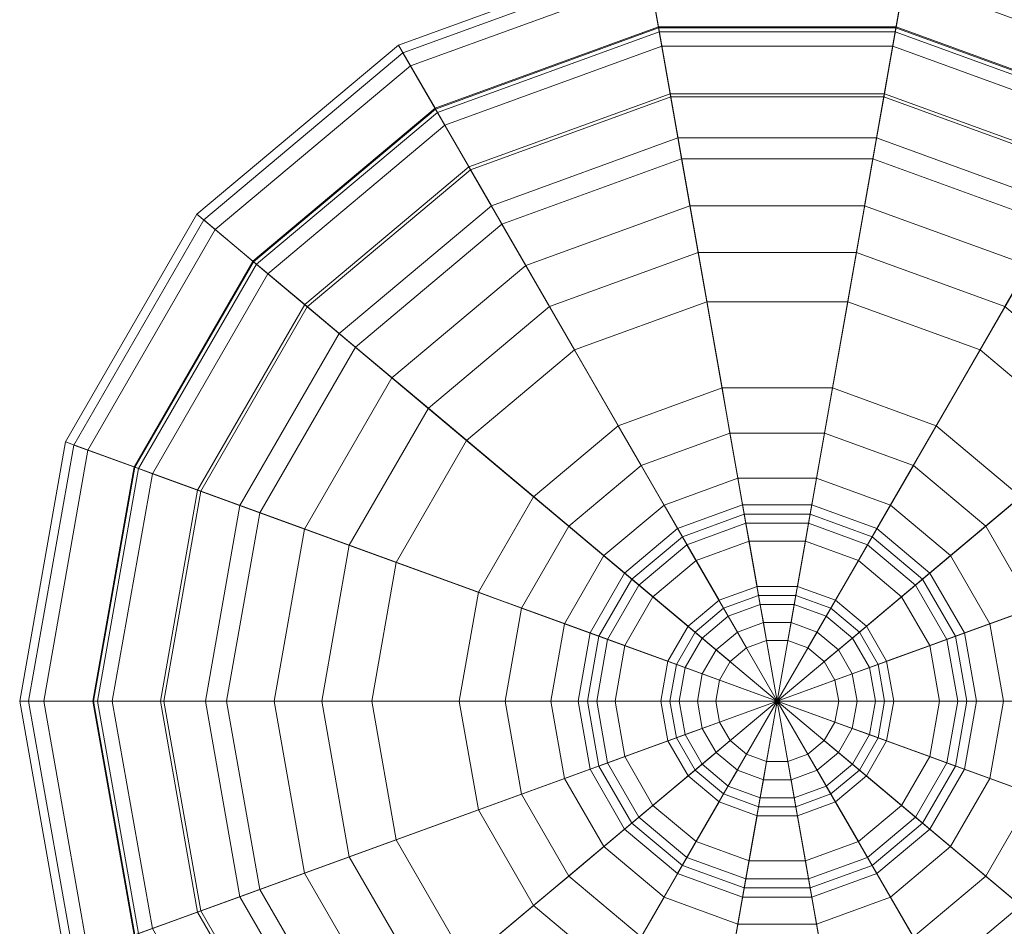
# Model space of a CAD drawing. Units: inches. Extents: x 375 to 1122, y 27 to 1069.
# Tile 42 of 155: x 717.909 to 719.669, y 298.684 to 300.305. Entities that reach past the tile are written whole.
import ezdxf

# ---------------------------------------------------------------- set-up
doc = ezdxf.new("R2010")
doc.units = ezdxf.units.IN
doc.layers.add('Furniture', color=30, linetype='Continuous', lineweight=18)

# ---------------------------------------------------------------- blocks, each defined once
blk = doc.blocks.new('A$C403C54AD')
for points in [[(1.180252, 0.891746, -0.031825), (1.180252, 0.857884, -0.028747), (1.180252, 0.857884, -0.028747), (1.16867, 0.889704, -0.031825)], [(1.191834, 0.889704, -0.031825), (1.180252, 0.857884, -0.028747), (1.180252, 0.857884, -0.028747), (1.180252, 0.891746, -0.031825)], [(1.16867, 0.889704, -0.031825), (1.180252, 0.857884, -0.028747), (1.180252, 0.857884, -0.028747), (1.158486, 0.883824, -0.031825)], [(1.202018, 0.883824, -0.031825), (1.180252, 0.857884, -0.028747), (1.180252, 0.857884, -0.028747), (1.191834, 0.889704, -0.031825)], [(1.158486, 0.883824, -0.031825), (1.180252, 0.857884, -0.028747), (1.180252, 0.857884, -0.028747), (1.150927, 0.874815, -0.031825)], [(1.209578, 0.874815, -0.031825), (1.180252, 0.857884, -0.028747), (1.180252, 0.857884, -0.028747), (1.202018, 0.883824, -0.031825)], [(1.171115, 0.868773, -0.02532), (1.160585, 0.881322, -0.028594), (1.153755, 0.873182, -0.028594), (1.167942, 0.864991, -0.02532)], [(1.192562, 0.864991, -0.02532), (1.206749, 0.873182, -0.028594), (1.199919, 0.881322, -0.028594), (1.189389, 0.868773, -0.02532)], [(1.180252, 0.878242, 0.061451), (1.180252, 0.868003, 0.054084), (1.176791, 0.867392, 0.054084), (1.173289, 0.877014, 0.061451)], [(1.187215, 0.877014, 0.061451), (1.183713, 0.867392, 0.054084), (1.180252, 0.868003, 0.054084), (1.180252, 0.878242, 0.061451)], [(1.1686, 0.87177, 0.063639), (1.164431, 0.876739, 0.073031), (1.158936, 0.87019, 0.073031), (1.164553, 0.866948, 0.063639)], [(1.173289, 0.877014, 0.061451), (1.176791, 0.867392, 0.054084), (1.173748, 0.865635, 0.054084), (1.167166, 0.873479, 0.061451)], [(1.193338, 0.873479, 0.061451), (1.186756, 0.865635, 0.054084), (1.183713, 0.867392, 0.054084), (1.187215, 0.877014, 0.061451)], [(1.180252, 0.866788, 0.057003), (1.180252, 0.876011, 0.063639), (1.174052, 0.874918, 0.063639), (1.177207, 0.866251, 0.057003)], [(1.183297, 0.866251, 0.057003), (1.186452, 0.874918, 0.063639), (1.180252, 0.876011, 0.063639), (1.180252, 0.866788, 0.057003)], [(1.153755, 0.873182, -0.028594), (1.150927, 0.874815, -0.031825), (1.146904, 0.863764, -0.031825), (1.15012, 0.863197, -0.028594)], [(1.150927, 0.874815, -0.031825), (1.180252, 0.857884, -0.028747), (1.180252, 0.857884, -0.028747), (1.146904, 0.863764, -0.031825)], [(1.15379, 0.873162, 0.131159), (1.151272, 0.874616, 0.117935), (1.147297, 0.863695, 0.117935), (1.15016, 0.86319, 0.131159)], [(1.151272, 0.874616, 0.117935), (1.151856, 0.874278, 0.089693), (1.147962, 0.863578, 0.089693), (1.147297, 0.863695, 0.117935)], [(1.177207, 0.866251, 0.057003), (1.174052, 0.874918, 0.063639), (1.1686, 0.87177, 0.063639), (1.174529, 0.864705, 0.057003)], [(1.2136, 0.863764, -0.031825), (1.180252, 0.857884, -0.028747), (1.180252, 0.857884, -0.028747), (1.209578, 0.874815, -0.031825)], [(1.185975, 0.864705, 0.057003), (1.191904, 0.87177, 0.063639), (1.186452, 0.874918, 0.063639), (1.183297, 0.866251, 0.057003)], [(1.151856, 0.874278, 0.089693), (1.156502, 0.871596, 0.071684), (1.153245, 0.862646, 0.071684), (1.147962, 0.863578, 0.089693)], [(1.167942, 0.864991, -0.02532), (1.153755, 0.873182, -0.028594), (1.15012, 0.863197, -0.028594), (1.166254, 0.860352, -0.02532)], [(1.167166, 0.873479, 0.061451), (1.173748, 0.865635, 0.054084), (1.171489, 0.862943, 0.054084), (1.162622, 0.868063, 0.061451)], [(1.197882, 0.868063, 0.061451), (1.189015, 0.862943, 0.054084), (1.186756, 0.865635, 0.054084), (1.193338, 0.873479, 0.061451)], [(1.158117, 0.870664, 0.140564), (1.15379, 0.873162, 0.131159), (1.15016, 0.86319, 0.131159), (1.155081, 0.862322, 0.140564)], [(1.153943, 0.873073, 0.117718), (1.156376, 0.871669, 0.130354), (1.153102, 0.862671, 0.130354), (1.150335, 0.863159, 0.117718)], [(1.154513, 0.872744, 0.090178), (1.153943, 0.873073, 0.117718), (1.150335, 0.863159, 0.117718), (1.150983, 0.863045, 0.090178)], [(1.158936, 0.87019, 0.073031), (1.154513, 0.872744, 0.090178), (1.150983, 0.863045, 0.090178), (1.156013, 0.862158, 0.073031)], [(1.156376, 0.871669, 0.130354), (1.160783, 0.869125, 0.140564), (1.158112, 0.861788, 0.140564), (1.153102, 0.862671, 0.130354)], [(1.156502, 0.871596, 0.071684), (1.162622, 0.868063, 0.061451), (1.160204, 0.861419, 0.061451), (1.153245, 0.862646, 0.071684)], [(1.174529, 0.864705, 0.057003), (1.1686, 0.87177, 0.063639), (1.164553, 0.866948, 0.063639), (1.172541, 0.862336, 0.057003)], [(1.187963, 0.862336, 0.057003), (1.195951, 0.866948, 0.063639), (1.191904, 0.87177, 0.063639), (1.185975, 0.864705, 0.057003)], [(1.176091, 0.869317, -0.022455), (1.17539, 0.871241, -0.02532), (1.171115, 0.868773, -0.02532), (1.172432, 0.867204, -0.022455)], [(1.188073, 0.867204, -0.022455), (1.189389, 0.868773, -0.02532), (1.185114, 0.871241, -0.02532), (1.184413, 0.869317, -0.022455)], [(1.160783, 0.869125, 0.140564), (1.158117, 0.870664, 0.140564), (1.155081, 0.862322, 0.140564), (1.158112, 0.861788, 0.140564)], [(1.164553, 0.866948, 0.063639), (1.158936, 0.87019, 0.073031), (1.156013, 0.862158, 0.073031), (1.1624, 0.861032, 0.063639)], [(1.180252, 0.865955, -0.020408), (1.180252, 0.87005, -0.022455), (1.176091, 0.869317, -0.022455), (1.177492, 0.865468, -0.020408)], [(1.183012, 0.865468, -0.020408), (1.184413, 0.869317, -0.022455), (1.180252, 0.87005, -0.022455), (1.180252, 0.865955, -0.020408)], [(1.177492, 0.865468, -0.020408), (1.176091, 0.869317, -0.022455), (1.172432, 0.867204, -0.022455), (1.175064, 0.864067, -0.020408)], [(1.18544, 0.864067, -0.020408), (1.188073, 0.867204, -0.022455), (1.184413, 0.869317, -0.022455), (1.183012, 0.865468, -0.020408)], [(1.172432, 0.867204, -0.022455), (1.171115, 0.868773, -0.02532), (1.167942, 0.864991, -0.02532), (1.169716, 0.863967, -0.022455)], [(1.190789, 0.863967, -0.022455), (1.192562, 0.864991, -0.02532), (1.189389, 0.868773, -0.02532), (1.188073, 0.867204, -0.022455)], [(1.162622, 0.868063, 0.061451), (1.171489, 0.862943, 0.054084), (1.170287, 0.859641, 0.054084), (1.160204, 0.861419, 0.061451)], [(1.180252, 0.868003, 0.054084), (1.180252, 0.863088, 0.053266), (1.178472, 0.862774, 0.053266), (1.176791, 0.867392, 0.054084)], [(1.183713, 0.867392, 0.054084), (1.182032, 0.862774, 0.053266), (1.180252, 0.863088, 0.053266), (1.180252, 0.868003, 0.054084)], [(1.2003, 0.861419, 0.061451), (1.190217, 0.859641, 0.054084), (1.189015, 0.862943, 0.054084), (1.197882, 0.868063, 0.061451)], [(1.175064, 0.864067, -0.020408), (1.172432, 0.867204, -0.022455), (1.169716, 0.863967, -0.022455), (1.173262, 0.861919, -0.020408)], [(1.176791, 0.867392, 0.054084), (1.178472, 0.862774, 0.053266), (1.176907, 0.861871, 0.053266), (1.173748, 0.865635, 0.054084)], [(1.186756, 0.865635, 0.054084), (1.183597, 0.861871, 0.053266), (1.182032, 0.862774, 0.053266), (1.183713, 0.867392, 0.054084)], [(1.187242, 0.861919, -0.020408), (1.190789, 0.863967, -0.022455), (1.188073, 0.867204, -0.022455), (1.18544, 0.864067, -0.020408)], [(1.172541, 0.862336, 0.057003), (1.164553, 0.866948, 0.063639), (1.1624, 0.861032, 0.063639), (1.171483, 0.85943, 0.057003)], [(1.180252, 0.857884, 0.055519), (1.180252, 0.866788, 0.057003), (1.177207, 0.866251, 0.057003), (1.180252, 0.857884, 0.055519)], [(1.180252, 0.857884, 0.055519), (1.183297, 0.866251, 0.057003), (1.180252, 0.866788, 0.057003), (1.180252, 0.857884, 0.055519)], [(1.189021, 0.85943, 0.057003), (1.198104, 0.861032, 0.063639), (1.195951, 0.866948, 0.063639), (1.187963, 0.862336, 0.057003)], [(1.180252, 0.857884, 0.055519), (1.177207, 0.866251, 0.057003), (1.174529, 0.864705, 0.057003), (1.180252, 0.857884, 0.055519)], [(1.180252, 0.866365, 0.0504), (1.180252, 0.862269, 0.048354), (1.178752, 0.862005, 0.048354), (1.177352, 0.865853, 0.0504)], [(1.180252, 0.865136, 0.052447), (1.180252, 0.866365, 0.0504), (1.177352, 0.865853, 0.0504), (1.177772, 0.864699, 0.052447)], [(1.183153, 0.865853, 0.0504), (1.181752, 0.862005, 0.048354), (1.180252, 0.862269, 0.048354), (1.180252, 0.866365, 0.0504)], [(1.182732, 0.864699, 0.052447), (1.183153, 0.865853, 0.0504), (1.180252, 0.866365, 0.0504), (1.180252, 0.865136, 0.052447)], [(1.180252, 0.857884, 0.055519), (1.185975, 0.864705, 0.057003), (1.183297, 0.866251, 0.057003), (1.180252, 0.857884, 0.055519)], [(1.177352, 0.865853, 0.0504), (1.178752, 0.862005, 0.048354), (1.177433, 0.861243, 0.048354), (1.174801, 0.86438, 0.0504)], [(1.177772, 0.864699, 0.052447), (1.177352, 0.865853, 0.0504), (1.174801, 0.86438, 0.0504), (1.175591, 0.863439, 0.052447)], [(1.180252, 0.862679, -0.015087), (1.180252, 0.865955, -0.020408), (1.177492, 0.865468, -0.020408), (1.178612, 0.862389, -0.015087)], [(1.181892, 0.862389, -0.015087), (1.183012, 0.865468, -0.020408), (1.180252, 0.865955, -0.020408), (1.180252, 0.862679, -0.015087)], [(1.185703, 0.86438, 0.0504), (1.183071, 0.861243, 0.048354), (1.181752, 0.862005, 0.048354), (1.183153, 0.865853, 0.0504)], [(1.184913, 0.863439, 0.052447), (1.185703, 0.86438, 0.0504), (1.183153, 0.865853, 0.0504), (1.182732, 0.864699, 0.052447)], [(1.173748, 0.865635, 0.054084), (1.176907, 0.861871, 0.053266), (1.175745, 0.860486, 0.053266), (1.171489, 0.862943, 0.054084)], [(1.178612, 0.862389, -0.015087), (1.177492, 0.865468, -0.020408), (1.175064, 0.864067, -0.020408), (1.17717, 0.861557, -0.015087)], [(1.183334, 0.861557, -0.015087), (1.18544, 0.864067, -0.020408), (1.183012, 0.865468, -0.020408), (1.181892, 0.862389, -0.015087)], [(1.189015, 0.862943, 0.054084), (1.184759, 0.860486, 0.053266), (1.183597, 0.861871, 0.053266), (1.186756, 0.865635, 0.054084)], [(1.169716, 0.863967, -0.022455), (1.167942, 0.864991, -0.02532), (1.166254, 0.860352, -0.02532), (1.16827, 0.859997, -0.022455)], [(1.180252, 0.863088, 0.053266), (1.180252, 0.865136, 0.052447), (1.177772, 0.864699, 0.052447), (1.178472, 0.862774, 0.053266)], [(1.182032, 0.862774, 0.053266), (1.182732, 0.864699, 0.052447), (1.180252, 0.865136, 0.052447), (1.180252, 0.863088, 0.053266)], [(1.180252, 0.857884, 0.055519), (1.174529, 0.864705, 0.057003), (1.172541, 0.862336, 0.057003), (1.180252, 0.857884, 0.055519)], [(1.174801, 0.86438, 0.0504), (1.177433, 0.861243, 0.048354), (1.176454, 0.860076, 0.048354), (1.172908, 0.862124, 0.0504)], [(1.175591, 0.863439, 0.052447), (1.174801, 0.86438, 0.0504), (1.172908, 0.862124, 0.0504), (1.173972, 0.86151, 0.052447)], [(1.178472, 0.862774, 0.053266), (1.177772, 0.864699, 0.052447), (1.175591, 0.863439, 0.052447), (1.176907, 0.861871, 0.053266)], [(1.180252, 0.857884, 0.055519), (1.187963, 0.862336, 0.057003), (1.185975, 0.864705, 0.057003), (1.180252, 0.857884, 0.055519)], [(1.183597, 0.861871, 0.053266), (1.184913, 0.863439, 0.052447), (1.182732, 0.864699, 0.052447), (1.182032, 0.862774, 0.053266)], [(1.187596, 0.862124, 0.0504), (1.18405, 0.860076, 0.048354), (1.183071, 0.861243, 0.048354), (1.185703, 0.86438, 0.0504)], [(1.186532, 0.86151, 0.052447), (1.187596, 0.862124, 0.0504), (1.185703, 0.86438, 0.0504), (1.184913, 0.863439, 0.052447)], [(1.173262, 0.861919, -0.020408), (1.169716, 0.863967, -0.022455), (1.16827, 0.859997, -0.022455), (1.172304, 0.859285, -0.020408)], [(1.17717, 0.861557, -0.015087), (1.175064, 0.864067, -0.020408), (1.173262, 0.861919, -0.020408), (1.1761, 0.860281, -0.015087)], [(1.184404, 0.860281, -0.015087), (1.187242, 0.861919, -0.020408), (1.18544, 0.864067, -0.020408), (1.183334, 0.861557, -0.015087)], [(1.1882, 0.859285, -0.020408), (1.192234, 0.859997, -0.022455), (1.190789, 0.863967, -0.022455), (1.187242, 0.861919, -0.020408)], [(1.15012, 0.863197, -0.028594), (1.146904, 0.863764, -0.031825), (1.146904, 0.852004, -0.031825), (1.15012, 0.852571, -0.028594)], [(1.146904, 0.863764, -0.031825), (1.180252, 0.857884, -0.028747), (1.180252, 0.857884, -0.028747), (1.146904, 0.852004, -0.031825)], [(1.15016, 0.86319, 0.131159), (1.147297, 0.863695, 0.117935), (1.147297, 0.852073, 0.117935), (1.15016, 0.852578, 0.131159)], [(1.147962, 0.863578, 0.089693), (1.153245, 0.862646, 0.071684), (1.153245, 0.853122, 0.071684), (1.147962, 0.85219, 0.089693)], [(1.2136, 0.852004, -0.031825), (1.180252, 0.857884, -0.028747), (1.180252, 0.857884, -0.028747), (1.2136, 0.863764, -0.031825)], [(1.166254, 0.860352, -0.02532), (1.15012, 0.863197, -0.028594), (1.15012, 0.852571, -0.028594), (1.166254, 0.855416, -0.02532)], [(1.155081, 0.862322, 0.140564), (1.15016, 0.86319, 0.131159), (1.15016, 0.852578, 0.131159), (1.155081, 0.853446, 0.140564)], [(1.150335, 0.863159, 0.117718), (1.153102, 0.862671, 0.130354), (1.153102, 0.853097, 0.130354), (1.150335, 0.852609, 0.117718)], [(1.150983, 0.863045, 0.090178), (1.150335, 0.863159, 0.117718), (1.150335, 0.852609, 0.117718), (1.150983, 0.852723, 0.090178)], [(1.176907, 0.861871, 0.053266), (1.175591, 0.863439, 0.052447), (1.173972, 0.86151, 0.052447), (1.175745, 0.860486, 0.053266)], [(1.184759, 0.860486, 0.053266), (1.186532, 0.86151, 0.052447), (1.184913, 0.863439, 0.052447), (1.183597, 0.861871, 0.053266)], [(1.156013, 0.862158, 0.073031), (1.150983, 0.863045, 0.090178), (1.150983, 0.852723, 0.090178), (1.156013, 0.85361, 0.073031)], [(1.153102, 0.862671, 0.130354), (1.158112, 0.861788, 0.140564), (1.158112, 0.85398, 0.140564), (1.153102, 0.853097, 0.130354)], [(1.153245, 0.862646, 0.071684), (1.160204, 0.861419, 0.061451), (1.160204, 0.854349, 0.061451), (1.153245, 0.853122, 0.071684)], [(1.171489, 0.862943, 0.054084), (1.175745, 0.860486, 0.053266), (1.175127, 0.858788, 0.053266), (1.170287, 0.859641, 0.054084)], [(1.180252, 0.86145, -0.006492), (1.180252, 0.862679, -0.015087), (1.178612, 0.862389, -0.015087), (1.179032, 0.861235, -0.006492)], [(1.181472, 0.861235, -0.006492), (1.181892, 0.862389, -0.015087), (1.180252, 0.862679, -0.015087), (1.180252, 0.86145, -0.006492)], [(1.190217, 0.859641, 0.054084), (1.185377, 0.858788, 0.053266), (1.184759, 0.860486, 0.053266), (1.189015, 0.862943, 0.054084)], [(1.158112, 0.861788, 0.140564), (1.155081, 0.862322, 0.140564), (1.155081, 0.853446, 0.140564), (1.158112, 0.85398, 0.140564)], [(1.180252, 0.857884, 0.055519), (1.172541, 0.862336, 0.057003), (1.171483, 0.85943, 0.057003), (1.180252, 0.857884, 0.055519)], [(1.179032, 0.861235, -0.006492), (1.178612, 0.862389, -0.015087), (1.17717, 0.861557, -0.015087), (1.17796, 0.860616, -0.006492)], [(1.180252, 0.862269, 0.048354), (1.180252, 0.860631, 0.041805), (1.179313, 0.860465, 0.041805), (1.178752, 0.862005, 0.048354)], [(1.180252, 0.857884, 0.055519), (1.189021, 0.85943, 0.057003), (1.187963, 0.862336, 0.057003), (1.180252, 0.857884, 0.055519)], [(1.181752, 0.862005, 0.048354), (1.181191, 0.860465, 0.041805), (1.180252, 0.860631, 0.041805), (1.180252, 0.862269, 0.048354)], [(1.182544, 0.860616, -0.006492), (1.183334, 0.861557, -0.015087), (1.181892, 0.862389, -0.015087), (1.181472, 0.861235, -0.006492)], [(1.1624, 0.861032, 0.063639), (1.156013, 0.862158, 0.073031), (1.156013, 0.85361, 0.073031), (1.1624, 0.854736, 0.063639)], [(1.173972, 0.86151, 0.052447), (1.172908, 0.862124, 0.0504), (1.1719, 0.859357, 0.0504), (1.17311, 0.859143, 0.052447)], [(1.172908, 0.862124, 0.0504), (1.176454, 0.860076, 0.048354), (1.175934, 0.858645, 0.048354), (1.1719, 0.859357, 0.0504)], [(1.1761, 0.860281, -0.015087), (1.173262, 0.861919, -0.020408), (1.172304, 0.859285, -0.020408), (1.17553, 0.858717, -0.015087)], [(1.178752, 0.862005, 0.048354), (1.179313, 0.860465, 0.041805), (1.178486, 0.859988, 0.041805), (1.177433, 0.861243, 0.048354)], [(1.183071, 0.861243, 0.048354), (1.182018, 0.859988, 0.041805), (1.181191, 0.860465, 0.041805), (1.181752, 0.862005, 0.048354)], [(1.188604, 0.859357, 0.0504), (1.18457, 0.858645, 0.048354), (1.18405, 0.860076, 0.048354), (1.187596, 0.862124, 0.0504)], [(1.184974, 0.858717, -0.015087), (1.1882, 0.859285, -0.020408), (1.187242, 0.861919, -0.020408), (1.184404, 0.860281, -0.015087)], [(1.187394, 0.859143, 0.052447), (1.188604, 0.859357, 0.0504), (1.187596, 0.862124, 0.0504), (1.186532, 0.86151, 0.052447)], [(1.160204, 0.861419, 0.061451), (1.170287, 0.859641, 0.054084), (1.170287, 0.856127, 0.054084), (1.160204, 0.854349, 0.061451)], [(1.175745, 0.860486, 0.053266), (1.173972, 0.86151, 0.052447), (1.17311, 0.859143, 0.052447), (1.175127, 0.858788, 0.053266)], [(1.17796, 0.860616, -0.006492), (1.17717, 0.861557, -0.015087), (1.1761, 0.860281, -0.015087), (1.177164, 0.859667, -0.006492)], [(1.180252, 0.860631, 0.041805), (1.180252, 0.86145, -0.006492), (1.179032, 0.861235, -0.006492), (1.179313, 0.860465, 0.041805)], [(1.181191, 0.860465, 0.041805), (1.181472, 0.861235, -0.006492), (1.180252, 0.86145, -0.006492), (1.180252, 0.860631, 0.041805)], [(1.18334, 0.859667, -0.006492), (1.184404, 0.860281, -0.015087), (1.183334, 0.861557, -0.015087), (1.182544, 0.860616, -0.006492)], [(1.185377, 0.858788, 0.053266), (1.187394, 0.859143, 0.052447), (1.186532, 0.86151, 0.052447), (1.184759, 0.860486, 0.053266)], [(1.2003, 0.854349, 0.061451), (1.190217, 0.856127, 0.054084), (1.190217, 0.859641, 0.054084), (1.2003, 0.861419, 0.061451)], [(1.171483, 0.85943, 0.057003), (1.1624, 0.861032, 0.063639), (1.1624, 0.854736, 0.063639), (1.171483, 0.856338, 0.057003)], [(1.177433, 0.861243, 0.048354), (1.178486, 0.859988, 0.041805), (1.177873, 0.859257, 0.041805), (1.176454, 0.860076, 0.048354)], [(1.179313, 0.860465, 0.041805), (1.179032, 0.861235, -0.006492), (1.17796, 0.860616, -0.006492), (1.178486, 0.859988, 0.041805)], [(1.182018, 0.859988, 0.041805), (1.182544, 0.860616, -0.006492), (1.181472, 0.861235, -0.006492), (1.181191, 0.860465, 0.041805)], [(1.18405, 0.860076, 0.048354), (1.182631, 0.859257, 0.041805), (1.182018, 0.859988, 0.041805), (1.183071, 0.861243, 0.048354)], [(1.189021, 0.856338, 0.057003), (1.198104, 0.854736, 0.063639), (1.198104, 0.861032, 0.063639), (1.189021, 0.85943, 0.057003)], [(1.178486, 0.859988, 0.041805), (1.17796, 0.860616, -0.006492), (1.177164, 0.859667, -0.006492), (1.177873, 0.859257, 0.041805)], [(1.182631, 0.859257, 0.041805), (1.18334, 0.859667, -0.006492), (1.182544, 0.860616, -0.006492), (1.182018, 0.859988, 0.041805)], [(1.16827, 0.859997, -0.022455), (1.166254, 0.860352, -0.02532), (1.166254, 0.855416, -0.02532), (1.16827, 0.855771, -0.022455)], [(1.172304, 0.859285, -0.020408), (1.16827, 0.859997, -0.022455), (1.16827, 0.855771, -0.022455), (1.172304, 0.856482, -0.020408)], [(1.177164, 0.859667, -0.006492), (1.1761, 0.860281, -0.015087), (1.17553, 0.858717, -0.015087), (1.17674, 0.858503, -0.006492)], [(1.176454, 0.860076, 0.048354), (1.177873, 0.859257, 0.041805), (1.177547, 0.858361, 0.041805), (1.175934, 0.858645, 0.048354)], [(1.18457, 0.858645, 0.048354), (1.182957, 0.858361, 0.041805), (1.182631, 0.859257, 0.041805), (1.18405, 0.860076, 0.048354)], [(1.183764, 0.858503, -0.006492), (1.184974, 0.858717, -0.015087), (1.184404, 0.860281, -0.015087), (1.18334, 0.859667, -0.006492)], [(1.1882, 0.856482, -0.020408), (1.192234, 0.855771, -0.022455), (1.192234, 0.859997, -0.022455), (1.1882, 0.859285, -0.020408)], [(1.170287, 0.859641, 0.054084), (1.175127, 0.858788, 0.053266), (1.175127, 0.85698, 0.053266), (1.170287, 0.856127, 0.054084)], [(1.177873, 0.859257, 0.041805), (1.177164, 0.859667, -0.006492), (1.17674, 0.858503, -0.006492), (1.177547, 0.858361, 0.041805)], [(1.182957, 0.858361, 0.041805), (1.183764, 0.858503, -0.006492), (1.18334, 0.859667, -0.006492), (1.182631, 0.859257, 0.041805)], [(1.190217, 0.856127, 0.054084), (1.185377, 0.85698, 0.053266), (1.185377, 0.858788, 0.053266), (1.190217, 0.859641, 0.054084)], [(1.180252, 0.857884, 0.055519), (1.171483, 0.85943, 0.057003), (1.171483, 0.856338, 0.057003), (1.180252, 0.857884, 0.055519)], [(1.17311, 0.859143, 0.052447), (1.1719, 0.859357, 0.0504), (1.1719, 0.856411, 0.0504), (1.17311, 0.856625, 0.052447)], [(1.1719, 0.859357, 0.0504), (1.175934, 0.858645, 0.048354), (1.175934, 0.857123, 0.048354), (1.1719, 0.856411, 0.0504)], [(1.17553, 0.858717, -0.015087), (1.172304, 0.859285, -0.020408), (1.172304, 0.856482, -0.020408), (1.17553, 0.857051, -0.015087)], [(1.175127, 0.858788, 0.053266), (1.17311, 0.859143, 0.052447), (1.17311, 0.856625, 0.052447), (1.175127, 0.85698, 0.053266)], [(1.180252, 0.857884, 0.055519), (1.189021, 0.856338, 0.057003), (1.189021, 0.85943, 0.057003), (1.180252, 0.857884, 0.055519)], [(1.188604, 0.856411, 0.0504), (1.18457, 0.857123, 0.048354), (1.18457, 0.858645, 0.048354), (1.188604, 0.859357, 0.0504)], [(1.184974, 0.857051, -0.015087), (1.1882, 0.856482, -0.020408), (1.1882, 0.859285, -0.020408), (1.184974, 0.858717, -0.015087)], [(1.185377, 0.85698, 0.053266), (1.187394, 0.856625, 0.052447), (1.187394, 0.859143, 0.052447), (1.185377, 0.858788, 0.053266)], [(1.187394, 0.856625, 0.052447), (1.188604, 0.856411, 0.0504), (1.188604, 0.859357, 0.0504), (1.187394, 0.859143, 0.052447)], [(1.17674, 0.858503, -0.006492), (1.17553, 0.858717, -0.015087), (1.17553, 0.857051, -0.015087), (1.17674, 0.857265, -0.006492)], [(1.183764, 0.857265, -0.006492), (1.184974, 0.857051, -0.015087), (1.184974, 0.858717, -0.015087), (1.183764, 0.858503, -0.006492)], [(1.175934, 0.858645, 0.048354), (1.177547, 0.858361, 0.041805), (1.177547, 0.857407, 0.041805), (1.175934, 0.857123, 0.048354)], [(1.177547, 0.858361, 0.041805), (1.17674, 0.858503, -0.006492), (1.17674, 0.857265, -0.006492), (1.177547, 0.857407, 0.041805)], [(1.18457, 0.857123, 0.048354), (1.182957, 0.857407, 0.041805), (1.182957, 0.858361, 0.041805), (1.18457, 0.858645, 0.048354)], [(1.182957, 0.857407, 0.041805), (1.183764, 0.857265, -0.006492), (1.183764, 0.858503, -0.006492), (1.182957, 0.858361, 0.041805)], [(1.146904, 0.852004, -0.031825), (1.180252, 0.857884, -0.028747), (1.180252, 0.857884, -0.028747), (1.150927, 0.840953, -0.031825)], [(1.150927, 0.840953, -0.031825), (1.180252, 0.857884, -0.028747), (1.180252, 0.857884, -0.028747), (1.158486, 0.831944, -0.031825)], [(1.158486, 0.831944, -0.031825), (1.180252, 0.857884, -0.028747), (1.180252, 0.857884, -0.028747), (1.16867, 0.826064, -0.031825)], [(1.16867, 0.826064, -0.031825), (1.180252, 0.857884, -0.028747), (1.180252, 0.857884, -0.028747), (1.180252, 0.824022, -0.031825)], [(1.180252, 0.857884, 0.055519), (1.171483, 0.856338, 0.057003), (1.172541, 0.853432, 0.057003), (1.180252, 0.857884, 0.055519)], [(1.180252, 0.857884, 0.055519), (1.172541, 0.853432, 0.057003), (1.174529, 0.851063, 0.057003), (1.180252, 0.857884, 0.055519)], [(1.180252, 0.857884, 0.055519), (1.174529, 0.851063, 0.057003), (1.177207, 0.849517, 0.057003), (1.180252, 0.857884, 0.055519)], [(1.180252, 0.857884, 0.055519), (1.177207, 0.849517, 0.057003), (1.180252, 0.84898, 0.057003), (1.180252, 0.857884, 0.055519)], [(1.180252, 0.857884, 0.055519), (1.187963, 0.853432, 0.057003), (1.189021, 0.856338, 0.057003), (1.180252, 0.857884, 0.055519)], [(1.180252, 0.857884, 0.055519), (1.185975, 0.851063, 0.057003), (1.187963, 0.853432, 0.057003), (1.180252, 0.857884, 0.055519)], [(1.180252, 0.857884, 0.055519), (1.183297, 0.849517, 0.057003), (1.185975, 0.851063, 0.057003), (1.180252, 0.857884, 0.055519)], [(1.180252, 0.857884, 0.055519), (1.180252, 0.84898, 0.057003), (1.183297, 0.849517, 0.057003), (1.180252, 0.857884, 0.055519)], [(1.209578, 0.840953, -0.031825), (1.180252, 0.857884, -0.028747), (1.180252, 0.857884, -0.028747), (1.2136, 0.852004, -0.031825)], [(1.202018, 0.831944, -0.031825), (1.180252, 0.857884, -0.028747), (1.180252, 0.857884, -0.028747), (1.209578, 0.840953, -0.031825)], [(1.191834, 0.826064, -0.031825), (1.180252, 0.857884, -0.028747), (1.180252, 0.857884, -0.028747), (1.202018, 0.831944, -0.031825)], [(1.180252, 0.824022, -0.031825), (1.180252, 0.857884, -0.028747), (1.180252, 0.857884, -0.028747), (1.191834, 0.826064, -0.031825)], [(1.175934, 0.857123, 0.048354), (1.177547, 0.857407, 0.041805), (1.177873, 0.856511, 0.041805), (1.176454, 0.855691, 0.048354)], [(1.177547, 0.857407, 0.041805), (1.17674, 0.857265, -0.006492), (1.177164, 0.856101, -0.006492), (1.177873, 0.856511, 0.041805)], [(1.18405, 0.855691, 0.048354), (1.182631, 0.856511, 0.041805), (1.182957, 0.857407, 0.041805), (1.18457, 0.857123, 0.048354)], [(1.182631, 0.856511, 0.041805), (1.18334, 0.856101, -0.006492), (1.183764, 0.857265, -0.006492), (1.182957, 0.857407, 0.041805)], [(1.170287, 0.856127, 0.054084), (1.175127, 0.85698, 0.053266), (1.175745, 0.855282, 0.053266), (1.171489, 0.852825, 0.054084)], [(1.1719, 0.856411, 0.0504), (1.175934, 0.857123, 0.048354), (1.176454, 0.855691, 0.048354), (1.172908, 0.853644, 0.0504)], [(1.17553, 0.857051, -0.015087), (1.172304, 0.856482, -0.020408), (1.173262, 0.853848, -0.020408), (1.1761, 0.855487, -0.015087)], [(1.175127, 0.85698, 0.053266), (1.17311, 0.856625, 0.052447), (1.173972, 0.854258, 0.052447), (1.175745, 0.855282, 0.053266)], [(1.17674, 0.857265, -0.006492), (1.17553, 0.857051, -0.015087), (1.1761, 0.855487, -0.015087), (1.177164, 0.856101, -0.006492)], [(1.18334, 0.856101, -0.006492), (1.184404, 0.855487, -0.015087), (1.184974, 0.857051, -0.015087), (1.183764, 0.857265, -0.006492)], [(1.187596, 0.853644, 0.0504), (1.18405, 0.855691, 0.048354), (1.18457, 0.857123, 0.048354), (1.188604, 0.856411, 0.0504)], [(1.184404, 0.855487, -0.015087), (1.187242, 0.853848, -0.020408), (1.1882, 0.856482, -0.020408), (1.184974, 0.857051, -0.015087)], [(1.184759, 0.855282, 0.053266), (1.186532, 0.854258, 0.052447), (1.187394, 0.856625, 0.052447), (1.185377, 0.85698, 0.053266)], [(1.189015, 0.852825, 0.054084), (1.184759, 0.855282, 0.053266), (1.185377, 0.85698, 0.053266), (1.190217, 0.856127, 0.054084)], [(1.172304, 0.856482, -0.020408), (1.16827, 0.855771, -0.022455), (1.169716, 0.851801, -0.022455), (1.173262, 0.853848, -0.020408)], [(1.17311, 0.856625, 0.052447), (1.1719, 0.856411, 0.0504), (1.172908, 0.853644, 0.0504), (1.173972, 0.854258, 0.052447)], [(1.176454, 0.855691, 0.048354), (1.177873, 0.856511, 0.041805), (1.178486, 0.85578, 0.041805), (1.177433, 0.854525, 0.048354)], [(1.177873, 0.856511, 0.041805), (1.177164, 0.856101, -0.006492), (1.17796, 0.855152, -0.006492), (1.178486, 0.85578, 0.041805)], [(1.183071, 0.854525, 0.048354), (1.182018, 0.85578, 0.041805), (1.182631, 0.856511, 0.041805), (1.18405, 0.855691, 0.048354)], [(1.182018, 0.85578, 0.041805), (1.182544, 0.855152, -0.006492), (1.18334, 0.856101, -0.006492), (1.182631, 0.856511, 0.041805)], [(1.186532, 0.854258, 0.052447), (1.187596, 0.853644, 0.0504), (1.188604, 0.856411, 0.0504), (1.187394, 0.856625, 0.052447)], [(1.187242, 0.853848, -0.020408), (1.190789, 0.851801, -0.022455), (1.192234, 0.855771, -0.022455), (1.1882, 0.856482, -0.020408)], [(1.160204, 0.854349, 0.061451), (1.170287, 0.856127, 0.054084), (1.171489, 0.852825, 0.054084), (1.162622, 0.847705, 0.061451)], [(1.171483, 0.856338, 0.057003), (1.1624, 0.854736, 0.063639), (1.164553, 0.84882, 0.063639), (1.172541, 0.853432, 0.057003)], [(1.177164, 0.856101, -0.006492), (1.1761, 0.855487, -0.015087), (1.17717, 0.854211, -0.015087), (1.17796, 0.855152, -0.006492)], [(1.182544, 0.855152, -0.006492), (1.183334, 0.854211, -0.015087), (1.184404, 0.855487, -0.015087), (1.18334, 0.856101, -0.006492)], [(1.187963, 0.853432, 0.057003), (1.195951, 0.84882, 0.063639), (1.198104, 0.854736, 0.063639), (1.189021, 0.856338, 0.057003)], [(1.197882, 0.847705, 0.061451), (1.189015, 0.852825, 0.054084), (1.190217, 0.856127, 0.054084), (1.2003, 0.854349, 0.061451)], [(1.16827, 0.855771, -0.022455), (1.166254, 0.855416, -0.02532), (1.167942, 0.850777, -0.02532), (1.169716, 0.851801, -0.022455)], [(1.172908, 0.853644, 0.0504), (1.176454, 0.855691, 0.048354), (1.177433, 0.854525, 0.048354), (1.174801, 0.851387, 0.0504)], [(1.177433, 0.854525, 0.048354), (1.178486, 0.85578, 0.041805), (1.179313, 0.855303, 0.041805), (1.178752, 0.853763, 0.048354)], [(1.178486, 0.85578, 0.041805), (1.17796, 0.855152, -0.006492), (1.179032, 0.854533, -0.006492), (1.179313, 0.855303, 0.041805)], [(1.181752, 0.853763, 0.048354), (1.181191, 0.855303, 0.041805), (1.182018, 0.85578, 0.041805), (1.183071, 0.854525, 0.048354)], [(1.181191, 0.855303, 0.041805), (1.181472, 0.854533, -0.006492), (1.182544, 0.855152, -0.006492), (1.182018, 0.85578, 0.041805)], [(1.185703, 0.851387, 0.0504), (1.183071, 0.854525, 0.048354), (1.18405, 0.855691, 0.048354), (1.187596, 0.853644, 0.0504)], [(1.166254, 0.855416, -0.02532), (1.15012, 0.852571, -0.028594), (1.153755, 0.842586, -0.028594), (1.167942, 0.850777, -0.02532)], [(1.171489, 0.852825, 0.054084), (1.175745, 0.855282, 0.053266), (1.176907, 0.853897, 0.053266), (1.173748, 0.850133, 0.054084)], [(1.1761, 0.855487, -0.015087), (1.173262, 0.853848, -0.020408), (1.175064, 0.851701, -0.020408), (1.17717, 0.854211, -0.015087)], [(1.175745, 0.855282, 0.053266), (1.173972, 0.854258, 0.052447), (1.175591, 0.852329, 0.052447), (1.176907, 0.853897, 0.053266)], [(1.17796, 0.855152, -0.006492), (1.17717, 0.854211, -0.015087), (1.178612, 0.853379, -0.015087), (1.179032, 0.854533, -0.006492)], [(1.178752, 0.853763, 0.048354), (1.179313, 0.855303, 0.041805), (1.180252, 0.855137, 0.041805), (1.180252, 0.853499, 0.048354)], [(1.179313, 0.855303, 0.041805), (1.179032, 0.854533, -0.006492), (1.180252, 0.854318, -0.006492), (1.180252, 0.855137, 0.041805)], [(1.180252, 0.853499, 0.048354), (1.180252, 0.855137, 0.041805), (1.181191, 0.855303, 0.041805), (1.181752, 0.853763, 0.048354)], [(1.180252, 0.855137, 0.041805), (1.180252, 0.854318, -0.006492), (1.181472, 0.854533, -0.006492), (1.181191, 0.855303, 0.041805)], [(1.181472, 0.854533, -0.006492), (1.181892, 0.853379, -0.015087), (1.183334, 0.854211, -0.015087), (1.182544, 0.855152, -0.006492)], [(1.183334, 0.854211, -0.015087), (1.18544, 0.851701, -0.020408), (1.187242, 0.853848, -0.020408), (1.184404, 0.855487, -0.015087)], [(1.183597, 0.853897, 0.053266), (1.184913, 0.852329, 0.052447), (1.186532, 0.854258, 0.052447), (1.184759, 0.855282, 0.053266)], [(1.186756, 0.850133, 0.054084), (1.183597, 0.853897, 0.053266), (1.184759, 0.855282, 0.053266), (1.189015, 0.852825, 0.054084)], [(1.1624, 0.854736, 0.063639), (1.156013, 0.85361, 0.073031), (1.158936, 0.845577, 0.073031), (1.164553, 0.84882, 0.063639)], [(1.153245, 0.853122, 0.071684), (1.160204, 0.854349, 0.061451), (1.162622, 0.847705, 0.061451), (1.156502, 0.844172, 0.071684)], [(1.173972, 0.854258, 0.052447), (1.172908, 0.853644, 0.0504), (1.174801, 0.851387, 0.0504), (1.175591, 0.852329, 0.052447)], [(1.174801, 0.851387, 0.0504), (1.177433, 0.854525, 0.048354), (1.178752, 0.853763, 0.048354), (1.177352, 0.849915, 0.0504)], [(1.179032, 0.854533, -0.006492), (1.178612, 0.853379, -0.015087), (1.180252, 0.853089, -0.015087), (1.180252, 0.854318, -0.006492)], [(1.180252, 0.854318, -0.006492), (1.180252, 0.853089, -0.015087), (1.181892, 0.853379, -0.015087), (1.181472, 0.854533, -0.006492)], [(1.183153, 0.849915, 0.0504), (1.181752, 0.853763, 0.048354), (1.183071, 0.854525, 0.048354), (1.185703, 0.851387, 0.0504)], [(1.184913, 0.852329, 0.052447), (1.185703, 0.851387, 0.0504), (1.187596, 0.853644, 0.0504), (1.186532, 0.854258, 0.052447)], [(1.153102, 0.853097, 0.130354), (1.158112, 0.85398, 0.140564), (1.160783, 0.846643, 0.140564), (1.156376, 0.844099, 0.130354)], [(1.158112, 0.85398, 0.140564), (1.155081, 0.853446, 0.140564), (1.158117, 0.845104, 0.140564), (1.160783, 0.846643, 0.140564)], [(1.173262, 0.853848, -0.020408), (1.169716, 0.851801, -0.022455), (1.172432, 0.848564, -0.022455), (1.175064, 0.851701, -0.020408)], [(1.173748, 0.850133, 0.054084), (1.176907, 0.853897, 0.053266), (1.178472, 0.852994, 0.053266), (1.176791, 0.848375, 0.054084)], [(1.17717, 0.854211, -0.015087), (1.175064, 0.851701, -0.020408), (1.177492, 0.8503, -0.020408), (1.178612, 0.853379, -0.015087)], [(1.176907, 0.853897, 0.053266), (1.175591, 0.852329, 0.052447), (1.177772, 0.851069, 0.052447), (1.178472, 0.852994, 0.053266)], [(1.181892, 0.853379, -0.015087), (1.183012, 0.8503, -0.020408), (1.18544, 0.851701, -0.020408), (1.183334, 0.854211, -0.015087)], [(1.182032, 0.852994, 0.053266), (1.182732, 0.851069, 0.052447), (1.184913, 0.852329, 0.052447), (1.183597, 0.853897, 0.053266)], [(1.183713, 0.848375, 0.054084), (1.182032, 0.852994, 0.053266), (1.183597, 0.853897, 0.053266), (1.186756, 0.850133, 0.054084)], [(1.18544, 0.851701, -0.020408), (1.188073, 0.848564, -0.022455), (1.190789, 0.851801, -0.022455), (1.187242, 0.853848, -0.020408)], [(1.155081, 0.853446, 0.140564), (1.15016, 0.852578, 0.131159), (1.15379, 0.842606, 0.131159), (1.158117, 0.845104, 0.140564)], [(1.156013, 0.85361, 0.073031), (1.150983, 0.852723, 0.090178), (1.154513, 0.843024, 0.090178), (1.158936, 0.845577, 0.073031)], [(1.172541, 0.853432, 0.057003), (1.164553, 0.84882, 0.063639), (1.1686, 0.843998, 0.063639), (1.174529, 0.851063, 0.057003)], [(1.177352, 0.849915, 0.0504), (1.178752, 0.853763, 0.048354), (1.180252, 0.853499, 0.048354), (1.180252, 0.849403, 0.0504)], [(1.178612, 0.853379, -0.015087), (1.177492, 0.8503, -0.020408), (1.180252, 0.849813, -0.020408), (1.180252, 0.853089, -0.015087)], [(1.180252, 0.849403, 0.0504), (1.180252, 0.853499, 0.048354), (1.181752, 0.853763, 0.048354), (1.183153, 0.849915, 0.0504)], [(1.180252, 0.853089, -0.015087), (1.180252, 0.849813, -0.020408), (1.183012, 0.8503, -0.020408), (1.181892, 0.853379, -0.015087)], [(1.185975, 0.851063, 0.057003), (1.191904, 0.843998, 0.063639), (1.195951, 0.84882, 0.063639), (1.187963, 0.853432, 0.057003)], [(1.147962, 0.85219, 0.089693), (1.153245, 0.853122, 0.071684), (1.156502, 0.844172, 0.071684), (1.151856, 0.84149, 0.089693)], [(1.150335, 0.852609, 0.117718), (1.153102, 0.853097, 0.130354), (1.156376, 0.844099, 0.130354), (1.153943, 0.842695, 0.117718)], [(1.176791, 0.848375, 0.054084), (1.178472, 0.852994, 0.053266), (1.180252, 0.85268, 0.053266), (1.180252, 0.847765, 0.054084)], [(1.178472, 0.852994, 0.053266), (1.177772, 0.851069, 0.052447), (1.180252, 0.850632, 0.052447), (1.180252, 0.85268, 0.053266)], [(1.180252, 0.85268, 0.053266), (1.180252, 0.850632, 0.052447), (1.182732, 0.851069, 0.052447), (1.182032, 0.852994, 0.053266)], [(1.180252, 0.847765, 0.054084), (1.180252, 0.85268, 0.053266), (1.182032, 0.852994, 0.053266), (1.183713, 0.848375, 0.054084)], [(1.15012, 0.852571, -0.028594), (1.146904, 0.852004, -0.031825), (1.150927, 0.840953, -0.031825), (1.153755, 0.842586, -0.028594)], [(1.15016, 0.852578, 0.131159), (1.147297, 0.852073, 0.117935), (1.151272, 0.841152, 0.117935), (1.15379, 0.842606, 0.131159)], [(1.150983, 0.852723, 0.090178), (1.150335, 0.852609, 0.117718), (1.153943, 0.842695, 0.117718), (1.154513, 0.843024, 0.090178)], [(1.162622, 0.847705, 0.061451), (1.171489, 0.852825, 0.054084), (1.173748, 0.850133, 0.054084), (1.167166, 0.842289, 0.061451)], [(1.193338, 0.842289, 0.061451), (1.186756, 0.850133, 0.054084), (1.189015, 0.852825, 0.054084), (1.197882, 0.847705, 0.061451)], [(1.147297, 0.852073, 0.117935), (1.147962, 0.85219, 0.089693), (1.151856, 0.84149, 0.089693), (1.151272, 0.841152, 0.117935)], [(1.175591, 0.852329, 0.052447), (1.174801, 0.851387, 0.0504), (1.177352, 0.849915, 0.0504), (1.177772, 0.851069, 0.052447)], [(1.182732, 0.851069, 0.052447), (1.183153, 0.849915, 0.0504), (1.185703, 0.851387, 0.0504), (1.184913, 0.852329, 0.052447)], [(1.169716, 0.851801, -0.022455), (1.167942, 0.850777, -0.02532), (1.171115, 0.846995, -0.02532), (1.172432, 0.848564, -0.022455)], [(1.175064, 0.851701, -0.020408), (1.172432, 0.848564, -0.022455), (1.176091, 0.846451, -0.022455), (1.177492, 0.8503, -0.020408)], [(1.183012, 0.8503, -0.020408), (1.184413, 0.846451, -0.022455), (1.188073, 0.848564, -0.022455), (1.18544, 0.851701, -0.020408)], [(1.188073, 0.848564, -0.022455), (1.189389, 0.846995, -0.02532), (1.192562, 0.850777, -0.02532), (1.190789, 0.851801, -0.022455)], [(1.167942, 0.850777, -0.02532), (1.153755, 0.842586, -0.028594), (1.160585, 0.834446, -0.028594), (1.171115, 0.846995, -0.02532)], [(1.174529, 0.851063, 0.057003), (1.1686, 0.843998, 0.063639), (1.174052, 0.84085, 0.063639), (1.177207, 0.849517, 0.057003)], [(1.177772, 0.851069, 0.052447), (1.177352, 0.849915, 0.0504), (1.180252, 0.849403, 0.0504), (1.180252, 0.850632, 0.052447)], [(1.180252, 0.850632, 0.052447), (1.180252, 0.849403, 0.0504), (1.183153, 0.849915, 0.0504), (1.182732, 0.851069, 0.052447)], [(1.183297, 0.849517, 0.057003), (1.186452, 0.84085, 0.063639), (1.191904, 0.843998, 0.063639), (1.185975, 0.851063, 0.057003)], [(1.189389, 0.846995, -0.02532), (1.199919, 0.834446, -0.028594), (1.206749, 0.842586, -0.028594), (1.192562, 0.850777, -0.02532)], [(1.177492, 0.8503, -0.020408), (1.176091, 0.846451, -0.022455), (1.180252, 0.845717, -0.022455), (1.180252, 0.849813, -0.020408)], [(1.180252, 0.849813, -0.020408), (1.180252, 0.845717, -0.022455), (1.184413, 0.846451, -0.022455), (1.183012, 0.8503, -0.020408)], [(1.167166, 0.842289, 0.061451), (1.173748, 0.850133, 0.054084), (1.176791, 0.848375, 0.054084), (1.173289, 0.838754, 0.061451)], [(1.187215, 0.838754, 0.061451), (1.183713, 0.848375, 0.054084), (1.186756, 0.850133, 0.054084), (1.193338, 0.842289, 0.061451)], [(1.177207, 0.849517, 0.057003), (1.174052, 0.84085, 0.063639), (1.180252, 0.839757, 0.063639), (1.180252, 0.84898, 0.057003)], [(1.180252, 0.84898, 0.057003), (1.180252, 0.839757, 0.063639), (1.186452, 0.84085, 0.063639), (1.183297, 0.849517, 0.057003)], [(1.164553, 0.84882, 0.063639), (1.158936, 0.845577, 0.073031), (1.164431, 0.839029, 0.073031), (1.1686, 0.843998, 0.063639)], [(1.172432, 0.848564, -0.022455), (1.171115, 0.846995, -0.02532), (1.17539, 0.844527, -0.02532), (1.176091, 0.846451, -0.022455)], [(1.184413, 0.846451, -0.022455), (1.185114, 0.844527, -0.02532), (1.189389, 0.846995, -0.02532), (1.188073, 0.848564, -0.022455)], [(1.173289, 0.838754, 0.061451), (1.176791, 0.848375, 0.054084), (1.180252, 0.847765, 0.054084), (1.180252, 0.837526, 0.061451)], [(1.180252, 0.837526, 0.061451), (1.180252, 0.847765, 0.054084), (1.183713, 0.848375, 0.054084), (1.187215, 0.838754, 0.061451)], [(1.156502, 0.844172, 0.071684), (1.162622, 0.847705, 0.061451), (1.167166, 0.842289, 0.061451), (1.162624, 0.836876, 0.071684)], [(1.171115, 0.846995, -0.02532), (1.160585, 0.834446, -0.028594), (1.169787, 0.829133, -0.028594), (1.17539, 0.844527, -0.02532)], [(1.185114, 0.844527, -0.02532), (1.190717, 0.829133, -0.028594), (1.199919, 0.834446, -0.028594), (1.189389, 0.846995, -0.02532)], [(1.156376, 0.844099, 0.130354), (1.160783, 0.846643, 0.140564), (1.165801, 0.840662, 0.140564), (1.162531, 0.836765, 0.130354)], [(1.160783, 0.846643, 0.140564), (1.158117, 0.845104, 0.140564), (1.163823, 0.838304, 0.140564), (1.165801, 0.840662, 0.140564)], [(1.176091, 0.846451, -0.022455), (1.17539, 0.844527, -0.02532), (1.180252, 0.84367, -0.02532), (1.180252, 0.845717, -0.022455)], [(1.180252, 0.845717, -0.022455), (1.180252, 0.84367, -0.02532), (1.185114, 0.844527, -0.02532), (1.184413, 0.846451, -0.022455)], [(1.158936, 0.845577, 0.073031), (1.154513, 0.843024, 0.090178), (1.161148, 0.835117, 0.090178), (1.164431, 0.839029, 0.073031)], [(1.158117, 0.845104, 0.140564), (1.15379, 0.842606, 0.131159), (1.160611, 0.834477, 0.131159), (1.163823, 0.838304, 0.140564)], [(1.151856, 0.84149, 0.089693), (1.156502, 0.844172, 0.071684), (1.162624, 0.836876, 0.071684), (1.159176, 0.832767, 0.089693)], [(1.17539, 0.844527, -0.02532), (1.169787, 0.829133, -0.028594), (1.180252, 0.827288, -0.028594), (1.180252, 0.84367, -0.02532)], [(1.180252, 0.84367, -0.02532), (1.180252, 0.827288, -0.028594), (1.190717, 0.829133, -0.028594), (1.185114, 0.844527, -0.02532)], [(1.153943, 0.842695, 0.117718), (1.156376, 0.844099, 0.130354), (1.162531, 0.836765, 0.130354), (1.160725, 0.834612, 0.117718)], [(1.1686, 0.843998, 0.063639), (1.164431, 0.839029, 0.073031), (1.171834, 0.834755, 0.073031), (1.174052, 0.84085, 0.063639)], [(1.186452, 0.84085, 0.063639), (1.18867, 0.834755, 0.073031), (1.196073, 0.839029, 0.073031), (1.191904, 0.843998, 0.063639)], [(1.154513, 0.843024, 0.090178), (1.153943, 0.842695, 0.117718), (1.160725, 0.834612, 0.117718), (1.161148, 0.835117, 0.090178)], [(1.153755, 0.842586, -0.028594), (1.150927, 0.840953, -0.031825), (1.158486, 0.831944, -0.031825), (1.160585, 0.834446, -0.028594)], [(1.15379, 0.842606, 0.131159), (1.151272, 0.841152, 0.117935), (1.158742, 0.83225, 0.117935), (1.160611, 0.834477, 0.131159)], [(1.162624, 0.836876, 0.071684), (1.167166, 0.842289, 0.061451), (1.173289, 0.838754, 0.061451), (1.170873, 0.832114, 0.071684)], [(1.189632, 0.832114, 0.071684), (1.187215, 0.838754, 0.061451), (1.193338, 0.842289, 0.061451), (1.19788, 0.836876, 0.071684)], [(1.151272, 0.841152, 0.117935), (1.151856, 0.84149, 0.089693), (1.159176, 0.832767, 0.089693), (1.158742, 0.83225, 0.117935)], [(1.162531, 0.836765, 0.130354), (1.165801, 0.840662, 0.140564), (1.172563, 0.836759, 0.140564), (1.170823, 0.831977, 0.130354)], [(1.165801, 0.840662, 0.140564), (1.163823, 0.838304, 0.140564), (1.17151, 0.833866, 0.140564), (1.172563, 0.836759, 0.140564)], [(1.174052, 0.84085, 0.063639), (1.171834, 0.834755, 0.073031), (1.180252, 0.833271, 0.073031), (1.180252, 0.839757, 0.063639)], [(1.180252, 0.839757, 0.063639), (1.180252, 0.833271, 0.073031), (1.18867, 0.834755, 0.073031), (1.186452, 0.84085, 0.063639)], [(1.187941, 0.836759, 0.140564), (1.188994, 0.833866, 0.140564), (1.196681, 0.838304, 0.140564), (1.194703, 0.840662, 0.140564)], [(1.189681, 0.831977, 0.130354), (1.187941, 0.836759, 0.140564), (1.194703, 0.840662, 0.140564), (1.197973, 0.836765, 0.130354)], [(1.164431, 0.839029, 0.073031), (1.161148, 0.835117, 0.090178), (1.170087, 0.829956, 0.090178), (1.171834, 0.834755, 0.073031)], [(1.18867, 0.834755, 0.073031), (1.190417, 0.829956, 0.090178), (1.199356, 0.835117, 0.090178), (1.196073, 0.839029, 0.073031)], [(1.170873, 0.832114, 0.071684), (1.173289, 0.838754, 0.061451), (1.180252, 0.837526, 0.061451), (1.180252, 0.83046, 0.071684)], [(1.180252, 0.83046, 0.071684), (1.180252, 0.837526, 0.061451), (1.187215, 0.838754, 0.061451), (1.189632, 0.832114, 0.071684)], [(1.163823, 0.838304, 0.140564), (1.160611, 0.834477, 0.131159), (1.169801, 0.829171, 0.131159), (1.17151, 0.833866, 0.140564)], [(1.188994, 0.833866, 0.140564), (1.190703, 0.829171, 0.131159), (1.199893, 0.834477, 0.131159), (1.196681, 0.838304, 0.140564)], [(1.159176, 0.832767, 0.089693), (1.162624, 0.836876, 0.071684), (1.170873, 0.832114, 0.071684), (1.169038, 0.827073, 0.089693)], [(1.160725, 0.834612, 0.117718), (1.162531, 0.836765, 0.130354), (1.170823, 0.831977, 0.130354), (1.169862, 0.829337, 0.117718)], [(1.170823, 0.831977, 0.130354), (1.172563, 0.836759, 0.140564), (1.180252, 0.835403, 0.140564), (1.180252, 0.830315, 0.130354)], [(1.172563, 0.836759, 0.140564), (1.17151, 0.833866, 0.140564), (1.180252, 0.832324, 0.140564), (1.180252, 0.835403, 0.140564)], [(1.180252, 0.835403, 0.140564), (1.180252, 0.832324, 0.140564), (1.188994, 0.833866, 0.140564), (1.187941, 0.836759, 0.140564)], [(1.180252, 0.830315, 0.130354), (1.180252, 0.835403, 0.140564), (1.187941, 0.836759, 0.140564), (1.189681, 0.831977, 0.130354)], [(1.191466, 0.827073, 0.089693), (1.189632, 0.832114, 0.071684), (1.19788, 0.836876, 0.071684), (1.201328, 0.832767, 0.089693)], [(1.190642, 0.829337, 0.117718), (1.189681, 0.831977, 0.130354), (1.197973, 0.836765, 0.130354), (1.199779, 0.834612, 0.117718)], [(1.161148, 0.835117, 0.090178), (1.160725, 0.834612, 0.117718), (1.169862, 0.829337, 0.117718), (1.170087, 0.829956, 0.090178)], [(1.160611, 0.834477, 0.131159), (1.158742, 0.83225, 0.117935), (1.168807, 0.826439, 0.117935), (1.169801, 0.829171, 0.131159)], [(1.171834, 0.834755, 0.073031), (1.170087, 0.829956, 0.090178), (1.180252, 0.828163, 0.090178), (1.180252, 0.833271, 0.073031)], [(1.180252, 0.833271, 0.073031), (1.180252, 0.828163, 0.090178), (1.190417, 0.829956, 0.090178), (1.18867, 0.834755, 0.073031)], [(1.160585, 0.834446, -0.028594), (1.158486, 0.831944, -0.031825), (1.16867, 0.826064, -0.031825), (1.169787, 0.829133, -0.028594)], [(1.17151, 0.833866, 0.140564), (1.169801, 0.829171, 0.131159), (1.180252, 0.827328, 0.131159), (1.180252, 0.832324, 0.140564)], [(1.180252, 0.832324, 0.140564), (1.180252, 0.827328, 0.131159), (1.190703, 0.829171, 0.131159), (1.188994, 0.833866, 0.140564)], [(1.158742, 0.83225, 0.117935), (1.159176, 0.832767, 0.089693), (1.169038, 0.827073, 0.089693), (1.168807, 0.826439, 0.117935)], [(1.169038, 0.827073, 0.089693), (1.170873, 0.832114, 0.071684), (1.180252, 0.83046, 0.071684), (1.180252, 0.825096, 0.089693)], [(1.169862, 0.829337, 0.117718), (1.170823, 0.831977, 0.130354), (1.180252, 0.830315, 0.130354), (1.180252, 0.827505, 0.117718)], [(1.180252, 0.825096, 0.089693), (1.180252, 0.83046, 0.071684), (1.189632, 0.832114, 0.071684), (1.191466, 0.827073, 0.089693)], [(1.180252, 0.827505, 0.117718), (1.180252, 0.830315, 0.130354), (1.189681, 0.831977, 0.130354), (1.190642, 0.829337, 0.117718)], [(1.170087, 0.829956, 0.090178), (1.169862, 0.829337, 0.117718), (1.180252, 0.827505, 0.117718), (1.180252, 0.828163, 0.090178)], [(1.180252, 0.828163, 0.090178), (1.180252, 0.827505, 0.117718), (1.190642, 0.829337, 0.117718), (1.190417, 0.829956, 0.090178)], [(1.169801, 0.829171, 0.131159), (1.168807, 0.826439, 0.117935), (1.180252, 0.824421, 0.117935), (1.180252, 0.827328, 0.131159)], [(1.180252, 0.827328, 0.131159), (1.180252, 0.824421, 0.117935), (1.191697, 0.826439, 0.117935), (1.190703, 0.829171, 0.131159)], [(1.169787, 0.829133, -0.028594), (1.16867, 0.826064, -0.031825), (1.180252, 0.824022, -0.031825), (1.180252, 0.827288, -0.028594)], [(1.180252, 0.827288, -0.028594), (1.180252, 0.824022, -0.031825), (1.191834, 0.826064, -0.031825), (1.190717, 0.829133, -0.028594)], [(1.168807, 0.826439, 0.117935), (1.169038, 0.827073, 0.089693), (1.180252, 0.825096, 0.089693), (1.180252, 0.824421, 0.117935)], [(1.180252, 0.824421, 0.117935), (1.180252, 0.825096, 0.089693), (1.191466, 0.827073, 0.089693), (1.191697, 0.826439, 0.117935)]]:
    blk.add_3dface(points)

msp = doc.modelspace()

# ---------------------------------------------------------------- block references
at = {"layer": 'Furniture', "xscale": 39.9918517141215, "yscale": 39.9918517141215, "zscale": 39.9918517141215, "rotation": 270}
msp.add_blockref('A$C403C54AD', (684.9549, 346.2875, 0.024), dxfattribs=at)

doc.saveas('drawing.dxf')
